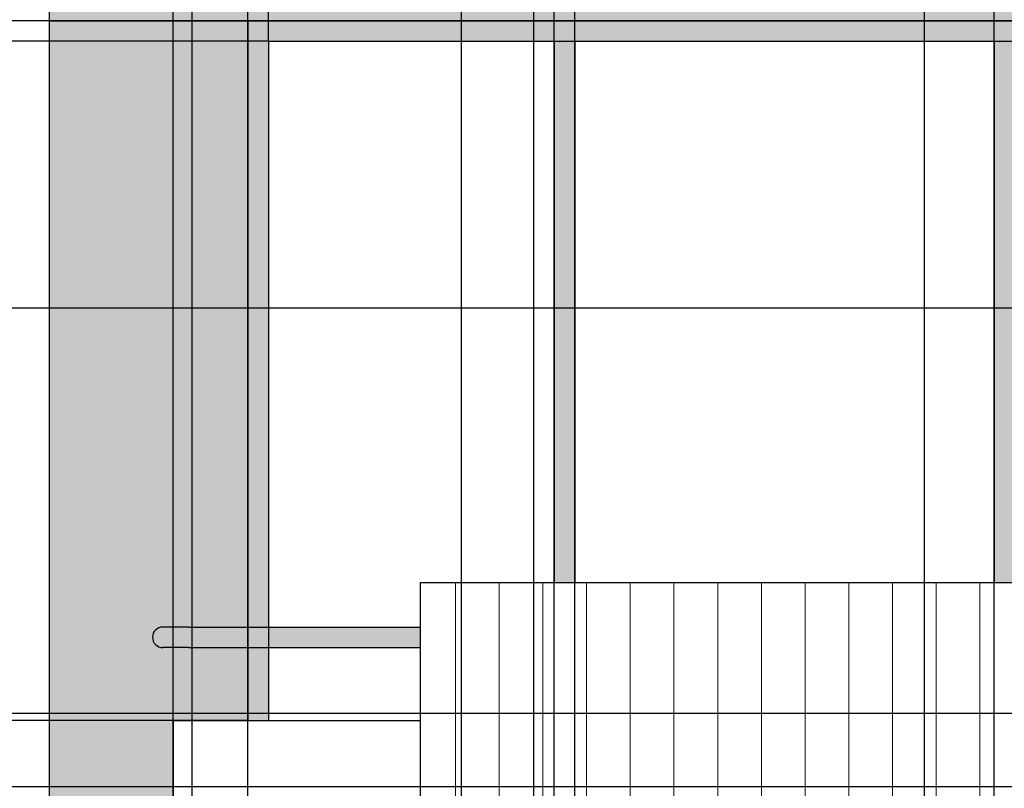
# Model space of a CAD drawing. Units: inches. Extents: x 241 to 943, y 109 to 1396.
# Tile 22 of 34: x 374 to 470, y 1103 to 1178. Entities that reach past the tile are written whole.
import ezdxf

# ---------------------------------------------------------------- set-up
doc = ezdxf.new("R2010")
doc.units = ezdxf.units.IN
doc.header["$MEASUREMENT"] = 0
for name, color, linetype, lineweight in [('A-ANNO-DIMS', 2, 'Continuous', 18), ('A-ELEV', 7, 'Continuous', 25), ('A-ELEV-SHAD', 9, 'Continuous', 13), ('A-GLAZ-PATT', 18, 'Continuous', 13), ('A-WALL-PATT', 8, 'Continuous', 13)]:
    doc.layers.add(name, color=color, linetype=linetype, lineweight=lineweight)
doc.styles.get("Standard").update_dxf_attribs({"font": 'arial.ttf'})
doc.dimstyles.get("Standard").update_dxf_attribs({"dimtxt": 1.4375, "dimasz": 0.18, "dimexe": 0.18, "dimexo": 0.0625, "dimgap": 0.09, "dimtad": 0, "dimtih": 1, "dimtoh": 1, "dimdec": 4, "dimzin": 0, "dimdsep": 46, "dimlunit": 4, "dimtxsty": 'Standard', "dimcen": 0.09, "dimadec": 0, "dimazin": 0, "dimtfac": 1, "dimtdec": 4, "dimtofl": 0, "dimtmove": 0, "dimatfit": 3, "dimfxl": 1, "dimtolj": 1, "dimtzin": 0, "dimarcsym": 0})

# ---------------------------------------------------------------- blocks, each defined once
blk = doc.blocks.new('BALCONY-RAIL')
for p, q in [((26.076, 26.374), (26.076, 52.061)), ((26.076, 52.061), (99.299, 52.061)), ((3.517, 47.727), (1, 47.727)), ((3.517, 47.727), (26.076, 47.727)), ((3.517, 45.727), (1, 45.727)), ((3.517, 45.727), (26.076, 45.727))]:
    blk.add_line(p, q)
blk.add_arc((1, 46.727), 1, 90, 270)
blk = doc.blocks.new('*D5')
at = {"layer": 'A-ANNO-DIMS', "color": 0, "lineweight": -2, "transparency": 16777216}
for p, q in [((303.236, 177.803), (303.236, 1395.045)), ((377.039, 177.76), (377.039, 1395.045)), ((303.416, 1394.865), (338.185, 1394.865)), ((376.859, 1394.865), (342.09, 1394.865))]:
    blk.add_line(p, q, dxfattribs=at)
at = {"layer": 'A-ANNO-DIMS', "color": 0, "transparency": 16777216}
for points in [[(303.416, 1394.895), (303.416, 1394.835), (303.236, 1394.865)], [(376.859, 1394.895), (376.859, 1394.835), (377.039, 1394.865)]]:
    blk.add_solid(points, dxfattribs=at)
at = {"layer": 'Defpoints', "color": 0, "transparency": 16777216}
for p in [(377.039, 1394.865), (303.236, 177.741), (377.039, 177.698)]:
    blk.add_point(p, dxfattribs=at)
at = {"layer": 'A-ANNO-DIMS', "color": 0, "transparency": 16777216, "insert": (340.137, 1394.865), "char_height": 1.4375, "attachment_point": 5}
blk.add_mtext('\\A1;73.8', dxfattribs=at)
blk = doc.blocks.new('*D7')
at = {"layer": 'A-ANNO-DIMS', "color": 0, "lineweight": -2, "transparency": 16777216}
for p, q in [((508.244, 1336.115), (244.306, 1336.115)), ((244.486, 1335.935), (244.486, 753.252)), ((244.486, 168.921), (244.486, 751.604)), ((303.173, 168.741), (244.306, 168.741))]:
    blk.add_line(p, q, dxfattribs=at)
at = {"layer": 'A-ANNO-DIMS', "color": 0, "transparency": 16777216}
for points in [[(244.456, 1335.935), (244.516, 1335.935), (244.486, 1336.115)], [(244.456, 168.921), (244.516, 168.921), (244.486, 168.741)]]:
    blk.add_solid(points, dxfattribs=at)
at = {"layer": 'Defpoints', "color": 0, "transparency": 16777216}
for p in [(244.486, 1336.115), (508.306, 1336.115), (303.236, 168.741)]:
    blk.add_point(p, dxfattribs=at)
at = {"layer": 'A-ANNO-DIMS', "color": 0, "transparency": 16777216, "insert": (244.486, 752.428), "char_height": 1.4375, "attachment_point": 5}
blk.add_mtext('\\A1;1167.4', dxfattribs=at)
blk = doc.blocks.new('*D8')
at = {"layer": 'A-ANNO-DIMS', "color": 0, "lineweight": -2, "transparency": 16777216}
for p, q in [((377.039, 396.941), (377.039, 1395.045)), ((390.895, 384.241), (390.895, 1395.045)), ((377.219, 1394.865), (380.961, 1394.865)), ((390.715, 1394.865), (386.973, 1394.865))]:
    blk.add_line(p, q, dxfattribs=at)
at = {"layer": 'A-ANNO-DIMS', "color": 0, "transparency": 16777216}
for points in [[(377.219, 1394.895), (377.219, 1394.835), (377.039, 1394.865)], [(390.715, 1394.895), (390.715, 1394.835), (390.895, 1394.865)]]:
    blk.add_solid(points, dxfattribs=at)
at = {"layer": 'Defpoints', "color": 0, "transparency": 16777216}
for p in [(390.895, 1394.865), (377.039, 396.878), (390.895, 384.178)]:
    blk.add_point(p, dxfattribs=at)
at = {"layer": 'A-ANNO-DIMS', "color": 0, "transparency": 16777216, "insert": (383.967, 1394.865), "char_height": 1.4375, "attachment_point": 5}
blk.add_mtext('\\A1;13.856', dxfattribs=at)
blk = doc.blocks.new('*D9')
at = {"layer": 'A-ANNO-DIMS', "color": 0, "lineweight": -2, "transparency": 16777216}
for p, q in [((390.895, 384.241), (390.895, 1395.045)), ((462.107, 384.241), (462.107, 1395.045)), ((391.075, 1394.865), (424.13, 1394.865)), ((461.927, 1394.865), (428.872, 1394.865))]:
    blk.add_line(p, q, dxfattribs=at)
at = {"layer": 'A-ANNO-DIMS', "color": 0, "transparency": 16777216}
for points in [[(391.075, 1394.895), (391.075, 1394.835), (390.895, 1394.865)], [(461.927, 1394.895), (461.927, 1394.835), (462.107, 1394.865)]]:
    blk.add_solid(points, dxfattribs=at)
at = {"layer": 'Defpoints', "color": 0, "transparency": 16777216}
for p in [(462.107, 1394.865), (390.895, 384.178), (462.107, 384.178)]:
    blk.add_point(p, dxfattribs=at)
at = {"layer": 'A-ANNO-DIMS', "color": 0, "transparency": 16777216, "insert": (426.501, 1394.865), "char_height": 1.4375, "attachment_point": 5}
blk.add_mtext('\\A1;71.21', dxfattribs=at)
blk = doc.blocks.new('*D10')
at = {"layer": 'A-ANNO-DIMS', "color": 0, "lineweight": -2, "transparency": 16777216}
for p, q in [((462.107, 384.241), (462.107, 1395.045)), ((479.596, 384.241), (479.596, 1395.045)), ((462.287, 1394.865), (468.402, 1394.865)), ((479.416, 1394.865), (473.301, 1394.865))]:
    blk.add_line(p, q, dxfattribs=at)
at = {"layer": 'A-ANNO-DIMS', "color": 0, "transparency": 16777216}
for points in [[(462.287, 1394.895), (462.287, 1394.835), (462.107, 1394.865)], [(479.416, 1394.895), (479.416, 1394.835), (479.596, 1394.865)]]:
    blk.add_solid(points, dxfattribs=at)
at = {"layer": 'Defpoints', "color": 0, "transparency": 16777216}
for p in [(479.596, 1394.865), (462.107, 384.178), (479.596, 384.178)]:
    blk.add_point(p, dxfattribs=at)
at = {"layer": 'A-ANNO-DIMS', "color": 0, "transparency": 16777216, "insert": (470.852, 1394.865), "char_height": 1.4375, "attachment_point": 5}
blk.add_mtext('\\A1;17.49', dxfattribs=at)
blk = doc.blocks.new('*D26')
at = {"layer": 'A-ANNO-DIMS', "color": 0, "lineweight": -2, "transparency": 16777216}
for p, q in [((376.977, 1177.538), (244.306, 1177.538)), ((244.486, 1177.358), (244.486, 1125.02)), ((244.486, 1071.034), (244.486, 1123.372)), ((376.977, 1070.854), (244.306, 1070.854))]:
    blk.add_line(p, q, dxfattribs=at)
at = {"layer": 'A-ANNO-DIMS', "color": 0, "transparency": 16777216}
for points in [[(244.456, 1177.358), (244.516, 1177.358), (244.486, 1177.538)], [(244.456, 1071.034), (244.516, 1071.034), (244.486, 1070.854)]]:
    blk.add_solid(points, dxfattribs=at)
at = {"layer": 'Defpoints', "color": 0, "transparency": 16777216}
for p in [(244.486, 1177.538), (377.039, 1177.538), (377.039, 1070.854)]:
    blk.add_point(p, dxfattribs=at)
at = {"layer": 'A-ANNO-DIMS', "color": 0, "transparency": 16777216, "insert": (244.486, 1124.196), "char_height": 1.4375, "attachment_point": 5}
blk.add_mtext('\\A1;106.68', dxfattribs=at)
blk = doc.blocks.new('*D27')
at = {"layer": 'A-ANNO-DIMS', "color": 0, "lineweight": -2, "transparency": 16777216}
for p, q in [((376.977, 1238.854), (244.306, 1238.854)), ((244.486, 1238.674), (244.486, 1209.02)), ((244.486, 1177.718), (244.486, 1207.372)), ((376.977, 1177.538), (244.306, 1177.538))]:
    blk.add_line(p, q, dxfattribs=at)
at = {"layer": 'A-ANNO-DIMS', "color": 0, "transparency": 16777216}
for points in [[(244.456, 1238.674), (244.516, 1238.674), (244.486, 1238.854)], [(244.456, 1177.718), (244.516, 1177.718), (244.486, 1177.538)]]:
    blk.add_solid(points, dxfattribs=at)
at = {"layer": 'Defpoints', "color": 0, "transparency": 16777216}
for p in [(244.486, 1238.854), (377.039, 1238.854), (377.039, 1177.538)]:
    blk.add_point(p, dxfattribs=at)
at = {"layer": 'A-ANNO-DIMS', "color": 0, "transparency": 16777216, "insert": (244.486, 1208.196), "char_height": 1.4375, "attachment_point": 5}
blk.add_mtext('\\A1;61.32', dxfattribs=at)
blk = doc.blocks.new('*D39')
at = {"layer": 'A-ANNO-DIMS', "color": 0, "lineweight": -2, "transparency": 16777216}
for p, q in [((388.98, 1109.492), (244.306, 1109.492)), ((244.486, 1109.312), (244.486, 1090.997)), ((244.486, 1071.034), (244.486, 1089.348)), ((388.98, 1070.854), (244.306, 1070.854))]:
    blk.add_line(p, q, dxfattribs=at)
at = {"layer": 'A-ANNO-DIMS', "color": 0, "transparency": 16777216}
for points in [[(244.456, 1109.312), (244.516, 1109.312), (244.486, 1109.492)], [(244.456, 1071.034), (244.516, 1071.034), (244.486, 1070.854)]]:
    blk.add_solid(points, dxfattribs=at)
at = {"layer": 'Defpoints', "color": 0, "transparency": 16777216}
for p in [(244.486, 1109.492), (389.043, 1109.492), (389.043, 1070.854)]:
    blk.add_point(p, dxfattribs=at)
at = {"layer": 'A-ANNO-DIMS', "color": 0, "transparency": 16777216, "insert": (244.486, 1090.173), "char_height": 1.4375, "attachment_point": 5}
blk.add_mtext('\\A1;38.64', dxfattribs=at)
blk = doc.blocks.new('*D40')
at = {"layer": 'A-ANNO-DIMS', "color": 0, "lineweight": -2, "transparency": 16777216}
for p, q in [((398.25, 1175.538), (244.306, 1175.538)), ((244.486, 1175.358), (244.486, 1143.339)), ((244.486, 1109.672), (244.486, 1141.691)), ((396.25, 1109.492), (244.306, 1109.492))]:
    blk.add_line(p, q, dxfattribs=at)
at = {"layer": 'A-ANNO-DIMS', "color": 0, "transparency": 16777216}
for points in [[(244.456, 1175.358), (244.516, 1175.358), (244.486, 1175.538)], [(244.456, 1109.672), (244.516, 1109.672), (244.486, 1109.492)]]:
    blk.add_solid(points, dxfattribs=at)
at = {"layer": 'Defpoints', "color": 0, "transparency": 16777216}
for p in [(244.486, 1175.538), (398.312, 1175.538), (396.312, 1109.492)]:
    blk.add_point(p, dxfattribs=at)
at = {"layer": 'A-ANNO-DIMS', "color": 0, "transparency": 16777216, "insert": (244.486, 1142.515), "char_height": 1.4375, "attachment_point": 5}
blk.add_mtext('\\A1;66.05', dxfattribs=at)
blk = doc.blocks.new('*D49')
at = {"layer": 'A-ANNO-DIMS', "color": 0, "lineweight": -2, "transparency": 16777216}
for p, q in [((766.241, 1177.538), (244.306, 1177.538)), ((244.486, 1177.358), (244.486, 1141.117)), ((244.486, 1103.228), (244.486, 1139.469)), ((766.241, 1103.048), (244.306, 1103.048))]:
    blk.add_line(p, q, dxfattribs=at)
at = {"layer": 'A-ANNO-DIMS', "color": 0, "transparency": 16777216}
for points in [[(244.456, 1177.358), (244.516, 1177.358), (244.486, 1177.538)], [(244.456, 1103.228), (244.516, 1103.228), (244.486, 1103.048)]]:
    blk.add_solid(points, dxfattribs=at)
at = {"layer": 'Defpoints', "color": 0, "transparency": 16777216}
for p in [(244.486, 1177.538), (766.304, 1177.538), (766.304, 1103.048)]:
    blk.add_point(p, dxfattribs=at)
at = {"layer": 'A-ANNO-DIMS', "color": 0, "transparency": 16777216, "insert": (244.486, 1140.293), "char_height": 1.4375, "attachment_point": 5}
blk.add_mtext('\\A1;74.49', dxfattribs=at)
blk = doc.blocks.new('*D59')
at = {"layer": 'A-ANNO-DIMS', "color": 0, "lineweight": -2, "transparency": 16777216}
for p, q in [((398.312, 1175.601), (398.312, 1395.045)), ((506.306, 1175.601), (506.306, 1395.045)), ((398.492, 1394.865), (450.698, 1394.865)), ((506.126, 1394.865), (453.921, 1394.865))]:
    blk.add_line(p, q, dxfattribs=at)
at = {"layer": 'A-ANNO-DIMS', "color": 0, "transparency": 16777216}
for points in [[(398.492, 1394.895), (398.492, 1394.835), (398.312, 1394.865)], [(506.126, 1394.895), (506.126, 1394.835), (506.306, 1394.865)]]:
    blk.add_solid(points, dxfattribs=at)
at = {"layer": 'Defpoints', "color": 0, "transparency": 16777216}
for p in [(506.306, 1394.865), (398.312, 1175.538), (506.306, 1175.538)]:
    blk.add_point(p, dxfattribs=at)
at = {"layer": 'A-ANNO-DIMS', "color": 0, "transparency": 16777216, "insert": (452.309, 1394.865), "char_height": 1.4375, "attachment_point": 5}
blk.add_mtext('\\A1;108', dxfattribs=at)
blk = doc.blocks.new('*D60')
at = {"layer": 'A-ANNO-DIMS', "color": 0, "lineweight": -2, "transparency": 16777216}
for p, q in [((377.039, 1177.601), (377.039, 1395.045)), ((398.312, 1175.601), (398.312, 1395.045)), ((377.219, 1394.865), (384.59, 1394.865)), ((398.132, 1394.865), (390.762, 1394.865))]:
    blk.add_line(p, q, dxfattribs=at)
at = {"layer": 'A-ANNO-DIMS', "color": 0, "transparency": 16777216}
for points in [[(377.219, 1394.895), (377.219, 1394.835), (377.039, 1394.865)], [(398.132, 1394.895), (398.132, 1394.835), (398.312, 1394.865)]]:
    blk.add_solid(points, dxfattribs=at)
at = {"layer": 'Defpoints', "color": 0, "transparency": 16777216}
for p in [(398.312, 1394.865), (377.039, 1177.538), (398.312, 1175.538)]:
    blk.add_point(p, dxfattribs=at)
at = {"layer": 'A-ANNO-DIMS', "color": 0, "transparency": 16777216, "insert": (387.676, 1394.865), "char_height": 1.4375, "attachment_point": 5}
blk.add_mtext('\\A1;21.273', dxfattribs=at)
blk = doc.blocks.new('*D61')
at = {"layer": 'A-ANNO-DIMS', "color": 0, "lineweight": -2, "transparency": 16777216}
for p, q in [((377.039, 400.892), (377.039, 1395.045)), ((424.109, 568.892), (424.109, 1395.045)), ((377.219, 1394.865), (398.03, 1394.865)), ((423.929, 1394.865), (403.118, 1394.865))]:
    blk.add_line(p, q, dxfattribs=at)
at = {"layer": 'A-ANNO-DIMS', "color": 0, "transparency": 16777216}
for points in [[(377.219, 1394.895), (377.219, 1394.835), (377.039, 1394.865)], [(423.929, 1394.895), (423.929, 1394.835), (424.109, 1394.865)]]:
    blk.add_solid(points, dxfattribs=at)
at = {"layer": 'Defpoints', "color": 0, "transparency": 16777216}
for p in [(424.109, 1394.865), (424.109, 568.829), (377.039, 400.829)]:
    blk.add_point(p, dxfattribs=at)
at = {"layer": 'A-ANNO-DIMS', "color": 0, "transparency": 16777216, "insert": (400.574, 1394.865), "char_height": 1.4375, "attachment_point": 5}
blk.add_mtext('\\A1;47.07', dxfattribs=at)
blk = doc.blocks.new('*D62')
at = {"layer": 'A-ANNO-DIMS', "color": 0, "lineweight": -2, "transparency": 16777216}
for p, q in [((424.109, 568.892), (424.109, 1395.045)), ((565.202, 568.892), (565.202, 1395.045)), ((424.289, 1394.865), (492.346, 1394.865)), ((565.022, 1394.865), (496.964, 1394.865))]:
    blk.add_line(p, q, dxfattribs=at)
at = {"layer": 'A-ANNO-DIMS', "color": 0, "transparency": 16777216}
for points in [[(424.289, 1394.895), (424.289, 1394.835), (424.109, 1394.865)], [(565.022, 1394.895), (565.022, 1394.835), (565.202, 1394.865)]]:
    blk.add_solid(points, dxfattribs=at)
at = {"layer": 'Defpoints', "color": 0, "transparency": 16777216}
for p in [(565.202, 1394.865), (424.109, 568.829), (565.202, 568.829)]:
    blk.add_point(p, dxfattribs=at)
at = {"layer": 'A-ANNO-DIMS', "color": 0, "transparency": 16777216, "insert": (494.655, 1394.865), "char_height": 1.4375, "attachment_point": 5}
blk.add_mtext('\\A1;141.1', dxfattribs=at)
blk = doc.blocks.new('*D65')
at = {"layer": 'A-ANNO-DIMS', "color": 0, "lineweight": -2, "transparency": 16777216}
for p, q in [((424.109, 700.854), (424.109, 1395.045)), ((592.954, 700.854), (592.954, 1395.045)), ((424.289, 1394.865), (505.52, 1394.865)), ((592.774, 1394.865), (511.543, 1394.865))]:
    blk.add_line(p, q, dxfattribs=at)
at = {"layer": 'A-ANNO-DIMS', "color": 0, "transparency": 16777216}
for points in [[(424.289, 1394.895), (424.289, 1394.835), (424.109, 1394.865)], [(592.774, 1394.895), (592.774, 1394.835), (592.954, 1394.865)]]:
    blk.add_solid(points, dxfattribs=at)
at = {"layer": 'Defpoints', "color": 0, "transparency": 16777216}
for p in [(592.954, 1394.865), (424.109, 700.791), (592.954, 700.791)]:
    blk.add_point(p, dxfattribs=at)
at = {"layer": 'A-ANNO-DIMS', "color": 0, "transparency": 16777216, "insert": (508.531, 1394.865), "char_height": 1.4375, "attachment_point": 5}
blk.add_mtext('\\A1;168.85', dxfattribs=at)
blk = doc.blocks.new('*D67')
at = {"layer": 'A-ANNO-DIMS', "color": 0, "lineweight": -2, "transparency": 16777216}
for p, q in [((389.043, 773.554), (389.043, 1395.045)), ((607.816, 773.554), (607.816, 1395.045)), ((389.223, 1394.865), (495.343, 1394.865)), ((607.636, 1394.865), (501.516, 1394.865))]:
    blk.add_line(p, q, dxfattribs=at)
at = {"layer": 'A-ANNO-DIMS', "color": 0, "transparency": 16777216}
for points in [[(389.223, 1394.895), (389.223, 1394.835), (389.043, 1394.865)], [(607.636, 1394.895), (607.636, 1394.835), (607.816, 1394.865)]]:
    blk.add_solid(points, dxfattribs=at)
at = {"layer": 'Defpoints', "color": 0, "transparency": 16777216}
for p in [(607.816, 1394.865), (389.043, 773.492), (607.816, 773.492)]:
    blk.add_point(p, dxfattribs=at)
at = {"layer": 'A-ANNO-DIMS', "color": 0, "transparency": 16777216, "insert": (498.43, 1394.865), "char_height": 1.4375, "attachment_point": 5}
blk.add_mtext('\\A1;218.77', dxfattribs=at)
blk = doc.blocks.new('*D69')
at = {"layer": 'A-ANNO-DIMS', "color": 0, "lineweight": -2, "transparency": 16777216}
for p, q in [((389.043, 941.554), (389.043, 1395.045)), ((568.135, 941.554), (568.135, 1395.045)), ((389.223, 1394.865), (476.28, 1394.865)), ((567.955, 1394.865), (480.898, 1394.865))]:
    blk.add_line(p, q, dxfattribs=at)
at = {"layer": 'A-ANNO-DIMS', "color": 0, "transparency": 16777216}
for points in [[(389.223, 1394.895), (389.223, 1394.835), (389.043, 1394.865)], [(567.955, 1394.895), (567.955, 1394.835), (568.135, 1394.865)]]:
    blk.add_solid(points, dxfattribs=at)
at = {"layer": 'Defpoints', "color": 0, "transparency": 16777216}
for p in [(568.135, 1394.865), (389.043, 941.492), (568.135, 941.492)]:
    blk.add_point(p, dxfattribs=at)
at = {"layer": 'A-ANNO-DIMS', "color": 0, "transparency": 16777216, "insert": (478.589, 1394.865), "char_height": 1.4375, "attachment_point": 5}
blk.add_mtext('\\A1;179.1', dxfattribs=at)
blk = doc.blocks.new('*D72')
at = {"layer": 'A-ANNO-DIMS', "color": 0, "lineweight": -2, "transparency": 16777216}
for p, q in [((389.043, 1109.554), (389.043, 1395.045)), ((486.342, 1109.554), (486.342, 1395.045)), ((389.223, 1394.865), (435.735, 1394.865)), ((486.162, 1394.865), (439.649, 1394.865))]:
    blk.add_line(p, q, dxfattribs=at)
at = {"layer": 'A-ANNO-DIMS', "color": 0, "transparency": 16777216}
for points in [[(389.223, 1394.895), (389.223, 1394.835), (389.043, 1394.865)], [(486.162, 1394.895), (486.162, 1394.835), (486.342, 1394.865)]]:
    blk.add_solid(points, dxfattribs=at)
at = {"layer": 'Defpoints', "color": 0, "transparency": 16777216}
for p in [(486.342, 1394.865), (389.043, 1109.492), (486.342, 1109.492)]:
    blk.add_point(p, dxfattribs=at)
at = {"layer": 'A-ANNO-DIMS', "color": 0, "transparency": 16777216, "insert": (437.692, 1394.865), "char_height": 1.4375, "attachment_point": 5}
blk.add_mtext('\\A1;97.3', dxfattribs=at)
blk = doc.blocks.new('*D89')
at = {"layer": 'A-ANNO-DIMS', "color": 0, "lineweight": -2, "transparency": 16777216}
for p, q in [((377.039, 841.601), (377.039, 1395.045)), ((617.759, 841.601), (617.759, 1395.045)), ((377.219, 1394.865), (494.321, 1394.865)), ((617.579, 1394.865), (500.478, 1394.865))]:
    blk.add_line(p, q, dxfattribs=at)
at = {"layer": 'A-ANNO-DIMS', "color": 0, "transparency": 16777216}
for points in [[(377.219, 1394.895), (377.219, 1394.835), (377.039, 1394.865)], [(617.579, 1394.895), (617.579, 1394.835), (617.759, 1394.865)]]:
    blk.add_solid(points, dxfattribs=at)
at = {"layer": 'Defpoints', "color": 0, "transparency": 16777216}
for p in [(617.759, 1394.865), (377.039, 841.538), (617.759, 841.538)]:
    blk.add_point(p, dxfattribs=at)
at = {"layer": 'A-ANNO-DIMS', "color": 0, "transparency": 16777216, "insert": (497.399, 1394.865), "char_height": 1.4375, "attachment_point": 5}
blk.add_mtext('\\A1;240.72', dxfattribs=at)
blk = doc.blocks.new('*D92')
at = {"layer": 'A-ANNO-DIMS', "color": 0, "lineweight": -2, "transparency": 16777216}
for p, q in [((508.244, 1336.115), (244.306, 1336.115)), ((244.486, 1335.935), (244.486, 1204.309)), ((244.486, 1071.034), (244.486, 1202.661)), ((508.244, 1070.854), (244.306, 1070.854))]:
    blk.add_line(p, q, dxfattribs=at)
at = {"layer": 'A-ANNO-DIMS', "color": 0, "transparency": 16777216}
for points in [[(244.456, 1335.935), (244.516, 1335.935), (244.486, 1336.115)], [(244.456, 1071.034), (244.516, 1071.034), (244.486, 1070.854)]]:
    blk.add_solid(points, dxfattribs=at)
at = {"layer": 'Defpoints', "color": 0, "transparency": 16777216}
for p in [(244.486, 1336.115), (508.306, 1336.115), (508.306, 1070.854)]:
    blk.add_point(p, dxfattribs=at)
at = {"layer": 'A-ANNO-DIMS', "color": 0, "transparency": 16777216, "insert": (244.486, 1203.485), "char_height": 1.4375, "attachment_point": 5}
blk.add_mtext('\\A1;265.26', dxfattribs=at)
blk = doc.blocks.new('*D99')
at = {"layer": 'A-ANNO-DIMS', "color": 0, "lineweight": -2, "transparency": 16777216}
for p, q in [((417.091, 181.712), (417.091, 1395.045)), ((667.393, 214.581), (667.393, 1395.045)), ((417.271, 1394.865), (539.159, 1394.865)), ((667.213, 1394.865), (545.326, 1394.865))]:
    blk.add_line(p, q, dxfattribs=at)
at = {"layer": 'A-ANNO-DIMS', "color": 0, "transparency": 16777216}
for points in [[(417.271, 1394.895), (417.271, 1394.835), (417.091, 1394.865)], [(667.213, 1394.895), (667.213, 1394.835), (667.393, 1394.865)]]:
    blk.add_solid(points, dxfattribs=at)
at = {"layer": 'Defpoints', "color": 0, "transparency": 16777216}
for p in [(667.393, 1394.865), (667.393, 214.519), (417.091, 181.649)]:
    blk.add_point(p, dxfattribs=at)
at = {"layer": 'A-ANNO-DIMS', "color": 0, "transparency": 16777216, "insert": (542.242, 1394.865), "char_height": 1.4375, "attachment_point": 5}
blk.add_mtext('\\A1;250.30', dxfattribs=at)
blk = doc.blocks.new('*D101')
at = {"layer": 'A-ANNO-DIMS', "color": 0, "lineweight": -2, "transparency": 16777216}
for p, q in [((396.312, 1009.601), (396.312, 1395.045)), ((426.117, 1007.601), (426.117, 1395.045)), ((396.492, 1394.865), (408.123, 1394.865)), ((425.937, 1394.865), (414.306, 1394.865))]:
    blk.add_line(p, q, dxfattribs=at)
at = {"layer": 'A-ANNO-DIMS', "color": 0, "transparency": 16777216}
for points in [[(396.492, 1394.895), (396.492, 1394.835), (396.312, 1394.865)], [(425.937, 1394.895), (425.937, 1394.835), (426.117, 1394.865)]]:
    blk.add_solid(points, dxfattribs=at)
at = {"layer": 'Defpoints', "color": 0, "transparency": 16777216}
for p in [(426.117, 1394.865), (396.312, 1009.538), (426.117, 1007.538)]:
    blk.add_point(p, dxfattribs=at)
at = {"layer": 'A-ANNO-DIMS', "color": 0, "transparency": 16777216, "insert": (411.215, 1394.865), "char_height": 1.4375, "attachment_point": 5}
blk.add_mtext('\\A1;29.805', dxfattribs=at)
blk = doc.blocks.new('*D102')
at = {"layer": 'A-ANNO-DIMS', "color": 0, "lineweight": -2, "transparency": 16777216}
for p, q in [((428.117, 1007.601), (428.117, 1395.045)), ((468.869, 1007.601), (468.869, 1395.045)), ((428.297, 1394.865), (445.944, 1394.865)), ((468.689, 1394.865), (451.043, 1394.865))]:
    blk.add_line(p, q, dxfattribs=at)
at = {"layer": 'A-ANNO-DIMS', "color": 0, "transparency": 16777216}
for points in [[(428.297, 1394.895), (428.297, 1394.835), (428.117, 1394.865)], [(468.689, 1394.895), (468.689, 1394.835), (468.869, 1394.865)]]:
    blk.add_solid(points, dxfattribs=at)
at = {"layer": 'Defpoints', "color": 0, "transparency": 16777216}
for p in [(468.869, 1394.865), (428.117, 1007.538), (468.869, 1007.538)]:
    blk.add_point(p, dxfattribs=at)
at = {"layer": 'A-ANNO-DIMS', "color": 0, "transparency": 16777216, "insert": (448.493, 1394.865), "char_height": 1.4375, "attachment_point": 5}
blk.add_mtext('\\A1;40.75', dxfattribs=at)
blk = doc.blocks.new('*D110')
at = {"layer": 'A-ANNO-DIMS', "color": 0, "lineweight": -2, "transparency": 16777216}
for p, q in [((535.89, 1149.577), (244.306, 1149.577)), ((244.486, 1149.397), (244.486, 1130.697)), ((244.486, 1110.349), (244.486, 1129.048)), ((535.89, 1110.169), (244.306, 1110.169))]:
    blk.add_line(p, q, dxfattribs=at)
at = {"layer": 'A-ANNO-DIMS', "color": 0, "transparency": 16777216}
for points in [[(244.456, 1149.397), (244.516, 1149.397), (244.486, 1149.577)], [(244.456, 1110.349), (244.516, 1110.349), (244.486, 1110.169)]]:
    blk.add_solid(points, dxfattribs=at)
at = {"layer": 'Defpoints', "color": 0, "transparency": 16777216}
for p in [(244.486, 1149.577), (535.952, 1149.577), (535.952, 1110.169)]:
    blk.add_point(p, dxfattribs=at)
at = {"layer": 'A-ANNO-DIMS', "color": 0, "transparency": 16777216, "insert": (244.486, 1129.873), "char_height": 1.4375, "attachment_point": 5}
blk.add_mtext('\\A1;39.41', dxfattribs=at)

msp = doc.modelspace()

# ---------------------------------------------------------------- hatches: boundary and pattern name
at = {"layer": 'A-ELEV-SHAD'}
h = msp.add_hatch(color=256, dxfattribs=at)
h.dxf.hatch_style = 1
h.paths.add_polyline_path([(508.3064, 1070.8538), (377.0391, 1070.8538), (377.0391, 1009.5382), (508.3064, 1009.5382)])
h.paths.add_polyline_path([(508.3064, 1238.8538), (377.0391, 1238.8538), (377.0391, 1177.5382), (508.3064, 1177.5382)])
h.paths.add_polyline_path([(581.3632, 902.8538), (568.1348, 902.8538), (553.5166, 902.8538), (377.0391, 902.8538), (377.0391, 841.5382), (553.5166, 841.5382), (564.8076, 841.5382), (581.3632, 841.5382)])
h.paths.add_polyline_path([(820.8374, 1275.9142), (747.7579, 1275.9142), (747.7579, 1238.8538), (820.8374, 1238.8538)])
h.paths.add_polyline_path([(820.8374, 1238.8538), (747.7579, 1238.8538), (747.9341, 1223.0633), (820.8374, 1223.0633)])
h.paths.add_polyline_path([(396.3125, 841.5382), (377.0391, 841.5382), (377.0391, 734.8538), (389.0429, 734.8538), (389.0429, 735.188), (389.0429, 773.4916), (396.3125, 773.4916), (396.3125, 780.5808), (390.5597, 780.5808), (388.0428, 780.5808, -1), (388.0428, 782.5808), (390.5597, 782.5808), (396.3125, 782.5808)])
h = msp.add_hatch(color=256, dxfattribs=at)
h.dxf.hatch_style = 1
h.paths.add_polyline_path([(537.4269, 698.7912), (534.1778, 698.7912), (534.1778, 659.3434), (537.4269, 659.3434)])
h.paths.add_polyline_path([(508.0803, 698.7912), (450.9259, 698.7912), (450.9259, 659.3434), (452.9259, 659.3434), (452.9259, 696.7912), (506.0803, 696.7912), (506.0803, 659.3434), (508.0803, 659.3434)])
h.paths.add_polyline_path([(481.5031, 696.7912), (479.5031, 696.7912), (479.5031, 659.3434), (481.5031, 659.3434)], flags=17)
h.paths.add_polyline_path([(481.5031, 657.3434), (479.5031, 657.3434), (479.5031, 653.3371), (481.5031, 653.3371)], flags=17)
h.paths.add_polyline_path([(508.0803, 657.3434), (506.0803, 657.3434), (506.0803, 653.3371), (452.9259, 653.3371), (452.9259, 657.3434), (450.9259, 657.3434), (450.9259, 651.3371), (508.0803, 651.3371)])
h.paths.add_polyline_path([(428.1173, 839.5382), (426.1173, 839.5382), (426.1173, 786.9154), (428.1173, 786.9154)], flags=17)
h.paths.add_polyline_path([(470.8692, 839.5382), (468.8692, 839.5382), (468.8692, 786.9154), (470.8692, 786.9154)], flags=17)
h.paths.add_polyline_path([(508.3064, 841.5382), (396.3125, 841.5382), (396.3125, 782.5808), (398.3125, 782.5808), (398.3125, 839.5382), (506.3064, 839.5382), (506.3064, 782.5808), (508.3064, 782.5808)])
h.paths.add_polyline_path([(398.3125, 780.5808), (396.3125, 780.5808), (396.3125, 773.4916), (398.3125, 773.4916)])
h.paths.add_polyline_path([(508.3064, 780.5808), (506.3064, 780.5808), (506.3064, 773.4916), (508.3064, 773.4916)])
h.paths.add_polyline_path([(715.6236, 841.5382), (678.2674, 841.5382), (678.2674, 734.8538), (715.6236, 734.8538)])
h.paths.add_polyline_path([(680.2674, 839.5382), (682.4526, 839.5382), (713.6236, 839.5382), (713.6236, 736.9235), (690.2047, 736.9235), (680.2674, 736.9235)], flags=16)
h.paths.add_polyline_path([(792.691, 841.5382), (747.7579, 841.5382), (747.7579, 734.8538), (754.5373, 734.8538), (754.5373, 736.9235), (754.5373, 839.5382), (756.7224, 839.5382), (787.8934, 839.5382), (787.8934, 765.9585), (792.691, 765.9585)])
h.paths.add_polyline_path([(659.2925, 1009.5382), (657.2925, 1009.5382), (657.2925, 902.8538), (659.2925, 902.8538)])
h.paths.add_polyline_path([(751.5078, 976.6275), (712.5839, 976.6275), (712.5839, 974.6275), (751.5078, 974.6275)])
h.paths.add_polyline_path([(470.8692, 1007.5382), (468.8692, 1007.5382), (468.8692, 954.9154), (470.8692, 954.9154)], flags=17)
h.paths.add_polyline_path([(508.3064, 1009.5382), (396.3125, 1009.5382), (396.3125, 950.5808), (398.3125, 950.5808), (398.3125, 1007.5382), (506.3064, 1007.5382), (506.3064, 950.5808), (508.3064, 950.5808)])
h.paths.add_polyline_path([(428.1173, 1007.5382), (426.1173, 1007.5382), (426.1173, 954.9154), (428.1173, 954.9154)], flags=17)
h.paths.add_polyline_path([(398.3125, 948.5808), (396.3125, 948.5808), (396.3125, 941.4916), (398.3125, 941.4916)])
h.paths.add_polyline_path([(508.3064, 948.5808), (506.3064, 948.5808), (506.3064, 941.4916), (508.3064, 941.4916)])
h.paths.add_polyline_path([(428.1173, 1175.5382), (426.1173, 1175.5382), (426.1173, 1122.9154), (428.1173, 1122.9154)], flags=17)
h.paths.add_polyline_path([(508.3064, 1177.5382), (396.3125, 1177.5382), (396.3125, 1118.5808), (398.3125, 1118.5808), (398.3125, 1175.5382), (506.3064, 1175.5382), (506.3064, 1118.5808), (506.8039, 1118.5808, -1), (506.8039, 1116.5808), (506.3064, 1116.5808), (506.3064, 1109.4916), (508.3064, 1109.4916)])
h.paths.add_polyline_path([(470.8692, 1175.5382), (468.8692, 1175.5382), (468.8692, 1122.9154), (470.8692, 1122.9154)], flags=17)
h.paths.add_polyline_path([(398.3125, 1116.5808), (396.3125, 1116.5808), (396.3125, 1109.4916), (398.3125, 1109.4916)], flags=17)
h.paths.add_polyline_path([(724.819, 1177.7336), (533.952, 1177.7336), (533.952, 1108.1686), (724.819, 1108.1686)])
h.paths.add_polyline_path([(535.952, 1175.7336), (722.819, 1175.7336), (722.819, 1110.1686), (535.952, 1110.1686)], flags=0)
h.paths.add_polyline_path([(622.521, 1136.0739), (643.4534, 1136.0739), (643.4534, 1134.0739), (622.521, 1134.0739)], flags=0)
h.paths.add_polyline_path([(722.819, 1175.7336), (535.952, 1175.7336), (535.952, 1110.1686), (722.819, 1110.1686)], flags=16)
h.paths.add_polyline_path([(565.947, 1151.5772), (535.952, 1151.5772), (535.952, 1149.5772), (565.947, 1149.5772)], flags=0)
h = msp.add_hatch(color=256, dxfattribs=at)
h.dxf.hatch_style = 1
h.paths.add_polyline_path([(396.3125, 1177.5382), (377.0391, 1177.5382), (377.0391, 1070.8538), (389.0429, 1070.8538), (389.0429, 1109.4916), (396.3125, 1109.4916), (396.3125, 1116.5808), (390.5597, 1116.5808), (388.0428, 1116.5808, -1), (388.0428, 1118.5808), (390.5597, 1118.5808), (396.3125, 1118.5808)])
at = {"layer": 'A-GLAZ-PATT'}
h = msp.add_hatch(dxfattribs=at)
h.set_pattern_fill('ANSI31', color=256, scale=34, angle=45)
h.paths.add_polyline_path([(486.3418, 786.9154), (413.1187, 786.9154), (413.1187, 761.2284), (486.3418, 761.2284)])
h.paths.add_polyline_path([(486.3418, 954.9154), (413.1187, 954.9154), (413.1187, 929.2284), (486.3418, 929.2284)])
h.paths.add_polyline_path([(462.1074, 289.6933), (390.895, 289.6933), (390.895, 277.4626), (390.895, 274.3507), (462.1074, 274.3507), (462.1074, 277.4626)])
h.paths.add_polyline_path([(500.3323, 289.6933), (479.596, 289.6933), (479.596, 274.3507), (500.3323, 274.3507)])
h.paths.add_polyline_path([(450.9259, 566.8295), (426.1086, 566.8295), (426.1086, 498.4395), (446.4348, 498.4395), (446.4348, 519.3754), (450.9259, 519.3754), (450.9259, 525.3816), (445.5808, 525.3816, -1), (445.5808, 527.3816), (450.9259, 527.3816)])
h.paths.add_polyline_path([(563.2023, 508.9074), (534.1778, 508.9074), (508.1906, 508.9074), (508.1906, 498.4395), (563.2023, 498.4395)])
h.paths.add_polyline_path([(747.6328, 700.7912), (712.0171, 700.7912), (712.0171, 628.4013), (747.6328, 628.4013)])
h.paths.add_polyline_path([(446.4348, 643.7483), (426.1086, 643.7483), (426.1086, 630.4013), (446.4348, 630.4013)])
h.paths.add_polyline_path([(564.8076, 841.5382), (553.5166, 841.5382), (508.3064, 841.5382), (508.3064, 782.5808), (564.8076, 782.5808)])
h.paths.add_polyline_path([(564.8076, 780.5808), (508.3064, 780.5808), (508.3064, 773.4916), (564.8076, 773.4916)])
h.paths.add_polyline_path([(792.691, 762.5799), (759.6248, 762.5799), (759.6248, 736.9235), (759.6248, 734.8538), (792.691, 734.8538)])
h.paths.add_polyline_path([(564.8076, 1009.5382), (553.5166, 1009.5382), (508.3064, 1009.5382), (508.3064, 950.5808), (562.3033, 950.5808, -1), (562.3033, 948.5808), (508.3064, 948.5808), (508.3064, 941.4916), (564.8076, 941.4916)])
h.paths.add_polyline_path([(486.3418, 1122.9154), (413.1187, 1122.9154), (413.1187, 1097.2284), (486.3418, 1097.2284)])
h = msp.add_hatch(color=256, dxfattribs=at)
h.dxf.hatch_style = 1
h.paths.add_polyline_path([(396.3125, 1118.5808), (390.5597, 1118.5808), (388.0428, 1118.5808, 1), (388.0428, 1116.5808), (390.5597, 1116.5808), (396.3125, 1116.5808)])
h.paths.add_polyline_path([(398.3125, 1118.5808), (396.3125, 1118.5808), (396.3125, 1116.5808), (398.3125, 1116.5808)])
h.paths.add_polyline_path([(413.1187, 1118.5808), (398.3125, 1118.5808), (398.3125, 1116.5808), (413.1187, 1116.5808)])
h.paths.add_polyline_path([(506.3064, 1118.5808), (486.3418, 1118.5808), (486.3418, 1116.5808), (506.3064, 1116.5808)])
h.paths.add_polyline_path([(506.8039, 1118.5808), (506.3064, 1118.5808), (506.3064, 1116.5808), (506.8039, 1116.5808, 1)])
h.paths.add_polyline_path([(396.3125, 950.5808), (390.5597, 950.5808), (388.0428, 950.5808, 1), (388.0428, 948.5808), (390.5597, 948.5808), (396.3125, 948.5808)])
h.paths.add_polyline_path([(398.3125, 950.5808), (396.3125, 950.5808), (396.3125, 948.5808), (398.3125, 948.5808)])
h.paths.add_polyline_path([(413.1187, 950.5808), (398.3125, 950.5808), (398.3125, 948.5808), (413.1187, 948.5808)])
h.paths.add_polyline_path([(506.3064, 950.5808), (486.3418, 950.5808), (486.3418, 948.5808), (506.3064, 948.5808)])
h.paths.add_polyline_path([(508.3064, 950.5808), (506.3064, 950.5808), (506.3064, 948.5808), (508.3064, 948.5808)])
h.paths.add_polyline_path([(562.3033, 950.5808), (508.3064, 950.5808), (508.3064, 948.5808), (562.3033, 948.5808, 1)])
h.paths.add_polyline_path([(396.3125, 782.5808), (390.5597, 782.5808), (388.0428, 782.5808, 1), (388.0428, 780.5808), (390.5597, 780.5808), (396.3125, 780.5808)])
h.paths.add_polyline_path([(398.3125, 782.5808), (396.3125, 782.5808), (396.3125, 780.5808), (398.3125, 780.5808)])
h.paths.add_polyline_path([(413.1187, 782.5808), (398.3125, 782.5808), (398.3125, 780.5808), (413.1187, 780.5808)])
h.paths.add_polyline_path([(506.3064, 782.5808), (486.3418, 782.5808), (486.3418, 780.5808), (506.3064, 780.5808)])
h.paths.add_polyline_path([(508.3064, 782.5808), (506.3064, 782.5808), (506.3064, 780.5808), (508.3064, 780.5808)])
h.paths.add_polyline_path([(564.8076, 782.5808), (508.3064, 782.5808), (508.3064, 780.5808), (564.8076, 780.5808)])
h.paths.add_polyline_path([(605.9087, 782.5808), (564.8076, 782.5808), (564.8076, 780.5808), (605.9087, 780.5808, 1)])
h.paths.add_polyline_path([(450.9259, 659.3434), (445.5808, 659.3434, 1), (445.5808, 657.3434), (450.9259, 657.3434)])
h.paths.add_polyline_path([(452.9259, 659.3434), (450.9259, 659.3434), (450.9259, 657.3434), (452.9259, 657.3434)])
h.paths.add_polyline_path([(506.0803, 659.3434), (452.9259, 659.3434), (452.9259, 657.3434), (506.0803, 657.3434)])
h.paths.add_polyline_path([(508.0803, 659.3434), (506.0803, 659.3434), (506.0803, 657.3434), (508.0803, 657.3434)])
h.paths.add_polyline_path([(563.2023, 659.3434), (537.4269, 659.3434), (537.4269, 657.3434), (563.2023, 657.3434)])
h.paths.add_polyline_path([(590.8792, 659.3434), (563.9297, 659.3434), (563.9297, 657.3434), (590.8792, 657.3434)])
h.paths.add_polyline_path([(563.9297, 659.3434), (563.2023, 659.3434), (563.2023, 657.3434), (563.9297, 657.3434)])
h.paths.add_polyline_path([(537.4269, 659.3434), (534.1778, 659.3434), (534.1778, 657.3434), (537.4269, 657.3434)])
h.paths.add_polyline_path([(534.1778, 659.3434), (508.0803, 659.3434), (508.0803, 657.3434), (534.1778, 657.3434)])
h.paths.add_polyline_path([(450.9259, 527.3816), (445.5808, 527.3816, 1), (445.5808, 525.3816), (450.9259, 525.3816)])
h.paths.add_polyline_path([(452.9259, 527.3816), (450.9259, 527.3816), (450.9259, 525.3816), (452.9259, 525.3816)])
h.paths.add_polyline_path([(479.5031, 527.3816), (452.9259, 527.3816), (452.9259, 525.3816), (479.5031, 525.3816)])
h.paths.add_polyline_path([(481.5031, 527.3816), (479.5031, 527.3816), (479.5031, 525.3816), (481.5031, 525.3816)])
h.paths.add_polyline_path([(506.0803, 527.3816), (481.5031, 527.3816), (481.5031, 525.3816), (506.0803, 525.3816)])
h.paths.add_polyline_path([(508.0803, 527.3816), (506.0803, 527.3816), (506.0803, 525.3816), (508.0803, 525.3816)])
h.paths.add_polyline_path([(563.2023, 527.3816), (508.0803, 527.3816), (508.0803, 525.3816), (563.2023, 525.3816)])
at = {"layer": 'A-WALL-PATT'}
h = msp.add_hatch(dxfattribs=at)
h.set_pattern_fill('GRATE', color=256, scale=150)
h.paths.add_polyline_path([(747.7579, 1238.8538), (747.7579, 1275.9142), (747.7579, 1336.1154), (508.3064, 1336.1154), (508.3064, 1275.9142), (508.3064, 1238.8538), (508.3064, 1177.5382), (508.3064, 1109.4916), (508.3064, 1070.8538), (553.5166, 1070.8538), (749.6328, 1070.8538)])
h.paths.add_polyline_path([(533.952, 1108.1686), (533.952, 1177.7336), (533.952, 1303.0286), (724.819, 1303.0286), (724.819, 1108.1686)], flags=16)
h.paths.add_polyline_path([(535.952, 1110.1686), (535.952, 1175.7336), (722.819, 1175.7336), (722.819, 1110.1686)], flags=0)
h.paths.add_polyline_path([(643.4534, 1134.0739), (622.521, 1134.0739), (622.521, 1136.0739), (643.4534, 1136.0739)], flags=0)
h.paths.add_polyline_path([(617.7594, 568.8295), (617.7594, 734.8538), (377.0391, 734.8538), (377.0391, 566.8538), (377.0391, 400.8295), (417.0913, 400.8295), (618.9643, 400.8295)])
h.paths.add_polyline_path([(424.1086, 496.4395), (424.1086, 568.8295), (565.2023, 568.8295), (565.2023, 496.4395)], flags=16)
h.paths.add_polyline_path([(426.1086, 498.4395), (426.1086, 566.8295), (563.2023, 566.8295), (563.2023, 508.9074), (563.2023, 498.4395)], flags=0)
h.paths.add_polyline_path([(508.0803, 508.9074), (508.0803, 519.3754), (450.9259, 519.3754), (450.9259, 525.3816), (445.5808, 525.3816, -1), (445.5808, 527.3816), (450.9259, 527.3816), (450.9259, 566.8295), (508.0803, 566.8295), (537.4269, 566.8295), (537.4269, 508.9074)], flags=0)
h.paths.add_polyline_path([(506.0803, 521.3754), (452.9259, 521.3754), (452.9259, 564.8295), (506.0803, 564.8295)], flags=0)
h.paths.add_polyline_path([(424.1086, 628.4013), (424.1086, 700.7912), (592.9542, 700.7912), (592.9542, 628.4013)], flags=16)
h.paths.add_polyline_path([(426.1086, 630.4013), (426.1086, 698.7912), (590.8792, 698.7912), (590.8792, 630.4013)], flags=0)
h.paths.add_polyline_path([(508.1906, 651.3371), (508.0803, 651.3371), (450.9259, 651.3371), (428.0291, 651.3371), (428.0291, 698.7912), (451.9767, 698.7912), (508.0803, 698.7912), (537.4269, 698.7912), (563.2023, 698.7912), (563.2023, 659.3434), (563.9297, 659.3434), (563.9297, 651.3371)], flags=0)
h.paths.add_polyline_path([(506.0803, 653.3371), (452.9259, 653.3371), (452.9259, 657.3434), (445.5808, 657.3434, -1), (445.5808, 659.3434), (452.9259, 659.3434), (452.9259, 696.7912), (506.0803, 696.7912)], flags=0)

# ---------------------------------------------------------------- linework, layer by layer
at = {"layer": 'A-ELEV'}
for p, q in [((377.0391, 1070.8538), (377.0391, 1238.8538)), ((377.0391, 1177.5382), (508.3064, 1177.5382)), ((396.3125, 1177.5382), (396.3125, 1109.4916)), ((398.3125, 1175.5382), (506.3064, 1175.5382)), ((398.3125, 1175.5382), (398.3125, 1109.4916)), ((426.1173, 1175.5382), (426.1173, 1122.9154)), ((428.1173, 1175.5382), (428.1173, 1122.9154)), ((468.8692, 1175.5382), (468.8692, 1122.9154)), ((389.0429, 1109.4916), (389.0429, 1070.8538)), ((389.0429, 1109.4916), (413.1187, 1109.4916))]:
    msp.add_line(p, q, dxfattribs=at)

# ---------------------------------------------------------------- block references
msp.add_blockref('BALCONY-RAIL', (387.043, 1070.854), dxfattribs=at)

# ---------------------------------------------------------------- dimensions: what is measured, and where the dimension line sits
at = {"layer": 'A-ANNO-DIMS'}
for base, p1, p2, override, picture, middle in [((377.0391, 1394.8654), (303.2358, 177.7407), (377.0391, 177.6977), {"dimdec": 1, "dimlfac": 1, "dimrnd": 0, "dimzin": 0, "dimdsep": 46, "dimlunit": 2}, '*D5', (340.1375, 1394.8654)), ((390.895, 1394.8654), (377.0391, 396.8782), (390.895, 384.1784), {"dimdec": 3, "dimlfac": 1, "dimrnd": 0, "dimzin": 0, "dimdsep": 46, "dimlunit": 2}, '*D8', (383.9671, 1394.8654)), ((398.3125, 1394.8654), (377.0391, 1177.5382), (398.3125, 1175.5382), {"dimdec": 3, "dimlfac": 1, "dimrnd": 0, "dimzin": 0, "dimdsep": 46, "dimlunit": 2}, '*D60', (387.6758, 1394.8654)), ((424.1086, 1394.8654), (377.0391, 400.8295), (424.1086, 568.8295), {"dimdec": 2, "dimlfac": 1, "dimrnd": 0, "dimzin": 0, "dimdsep": 46, "dimlunit": 2}, '*D61', (400.5739, 1394.8654)), ((617.7594, 1394.8654), (377.0391, 841.5382), (617.7594, 841.5382), {"dimdec": 2, "dimlfac": 1, "dimrnd": 0, "dimzin": 0, "dimdsep": 46, "dimlunit": 2}, '*D89', (497.3993, 1394.8654)), ((607.8162, 1394.8654), (389.0429, 773.4916), (607.8162, 773.4916), {"dimdec": 2, "dimlfac": 1, "dimrnd": 0, "dimzin": 0, "dimdsep": 46, "dimlunit": 2}, '*D67', (498.4295, 1394.8654)), ((568.1348, 1394.8654), (389.0429, 941.4916), (568.1348, 941.4916), {"dimdec": 1, "dimlfac": 1, "dimrnd": 0, "dimzin": 0, "dimdsep": 46, "dimlunit": 2}, '*D69', (478.5888, 1394.8654)), ((486.3418, 1394.8654), (389.0429, 1109.4916), (486.3418, 1109.4916), {"dimdec": 1, "dimlfac": 1, "dimrnd": 0, "dimzin": 0, "dimdsep": 46, "dimlunit": 2}, '*D72', (437.6924, 1394.8654)), ((462.1074, 1394.8654), (390.895, 384.1784), (462.1074, 384.1784), {"dimdec": 2, "dimlfac": 1, "dimrnd": 0, "dimzin": 0, "dimdsep": 46, "dimlunit": 2}, '*D9', (426.5012, 1394.8654)), ((426.1173, 1394.8654), (396.3125, 1009.5382), (426.1173, 1007.5382), {"dimdec": 3, "dimlfac": 1, "dimrnd": 0, "dimzin": 0, "dimdsep": 46, "dimlunit": 2}, '*D101', (411.2149, 1394.8654)), ((506.3064, 1394.8654), (398.3125, 1175.5382), (506.3064, 1175.5382), {"dimdec": 0, "dimlfac": 1, "dimrnd": 0, "dimzin": 0, "dimdsep": 46, "dimlunit": 2}, '*D59', (452.3095, 1394.8654)), ((667.3935, 1394.8654), (417.0913, 181.649), (667.3935, 214.5189), {"dimdec": 2, "dimlfac": 1, "dimrnd": 0, "dimzin": 0, "dimdsep": 46, "dimlunit": 2}, '*D99', (542.2424, 1394.8654)), ((565.2023, 1394.8654), (424.1086, 568.8295), (565.2023, 568.8295), {"dimdec": 1, "dimlfac": 1, "dimrnd": 0, "dimzin": 0, "dimdsep": 46, "dimlunit": 2}, '*D62', (494.6554, 1394.8654)), ((592.9542, 1394.8654), (424.1086, 700.7912), (592.9542, 700.7912), {"dimdec": 2, "dimlfac": 1, "dimrnd": 0, "dimzin": 0, "dimdsep": 46, "dimlunit": 2}, '*D65', (508.5314, 1394.8654)), ((468.8692, 1394.8654), (428.1173, 1007.5382), (468.8692, 1007.5382), {"dimdec": 2, "dimlfac": 1, "dimrnd": 0, "dimzin": 0, "dimdsep": 46, "dimlunit": 2}, '*D102', (448.4933, 1394.8654)), ((479.596, 1394.8654), (462.1074, 384.1784), (479.596, 384.1784), {"dimdec": 2, "dimlfac": 1, "dimrnd": 0, "dimzin": 0, "dimdsep": 46, "dimlunit": 2}, '*D10', (470.8517, 1394.8654))]:
    dim = msp.add_linear_dim(base=base, p1=p1, p2=p2, dimstyle='Standard', override=override, dxfattribs=at)
    dim.commit()
    dim.dimension.update_dxf_attribs({"geometry": picture, "text_midpoint": middle})
for base, p1, p2, override, picture, middle in [((244.4858, 1336.1154), (303.2358, 168.7407), (508.3064, 1336.1154), {"dimdec": 1, "dimlfac": 1, "dimrnd": 0, "dimzin": 0, "dimdsep": 46, "dimlunit": 2}, '*D7', (244.4858, 752.4281)), ((244.4858, 1336.1154), (508.3064, 1070.8538), (508.3064, 1336.1154), {"dimdec": 2, "dimlfac": 1, "dimrnd": 0, "dimzin": 0, "dimdsep": 46, "dimlunit": 2}, '*D92', (244.4858, 1203.4846)), ((244.4858, 1238.8538), (377.0391, 1177.5382), (377.0391, 1238.8538), {"dimdec": 2, "dimlfac": 1, "dimrnd": 0, "dimzin": 0, "dimdsep": 46, "dimlunit": 2}, '*D27', (244.4858, 1208.196)), ((244.4858, 1177.5382), (377.0391, 1070.8538), (377.0391, 1177.5382), {"dimdec": 2, "dimlfac": 1, "dimrnd": 0, "dimzin": 0, "dimdsep": 46, "dimlunit": 2}, '*D26', (244.4858, 1124.196)), ((244.4858, 1177.5382), (766.3038, 1103.0477), (766.3038, 1177.5382), {"dimdec": 2, "dimlfac": 1, "dimrnd": 0, "dimzin": 0, "dimdsep": 46, "dimlunit": 2}, '*D49', (244.4858, 1140.2929)), ((244.4858, 1175.5382), (396.3125, 1109.4916), (398.3125, 1175.5382), {"dimdec": 2, "dimlfac": 1, "dimrnd": 0, "dimzin": 0, "dimdsep": 46, "dimlunit": 2}, '*D40', (244.4858, 1142.5149)), ((244.4858, 1149.5772), (535.952, 1110.1686), (535.952, 1149.5772), {"dimdec": 2, "dimlfac": 1, "dimrnd": 0, "dimzin": 0, "dimdsep": 46, "dimlunit": 2}, '*D110', (244.4858, 1129.8729)), ((244.4858, 1109.4916), (389.0429, 1070.8538), (389.0429, 1109.4916), {"dimdec": 2, "dimlfac": 1, "dimrnd": 0, "dimzin": 0, "dimdsep": 46, "dimlunit": 2}, '*D39', (244.4858, 1090.1727))]:
    dim = msp.add_linear_dim(base=base, p1=p1, p2=p2, angle=90, dimstyle='Standard', override=override, dxfattribs=at)
    dim.commit()
    dim.dimension.update_dxf_attribs({"geometry": picture, "text_midpoint": middle})

doc.saveas('drawing.dxf')
